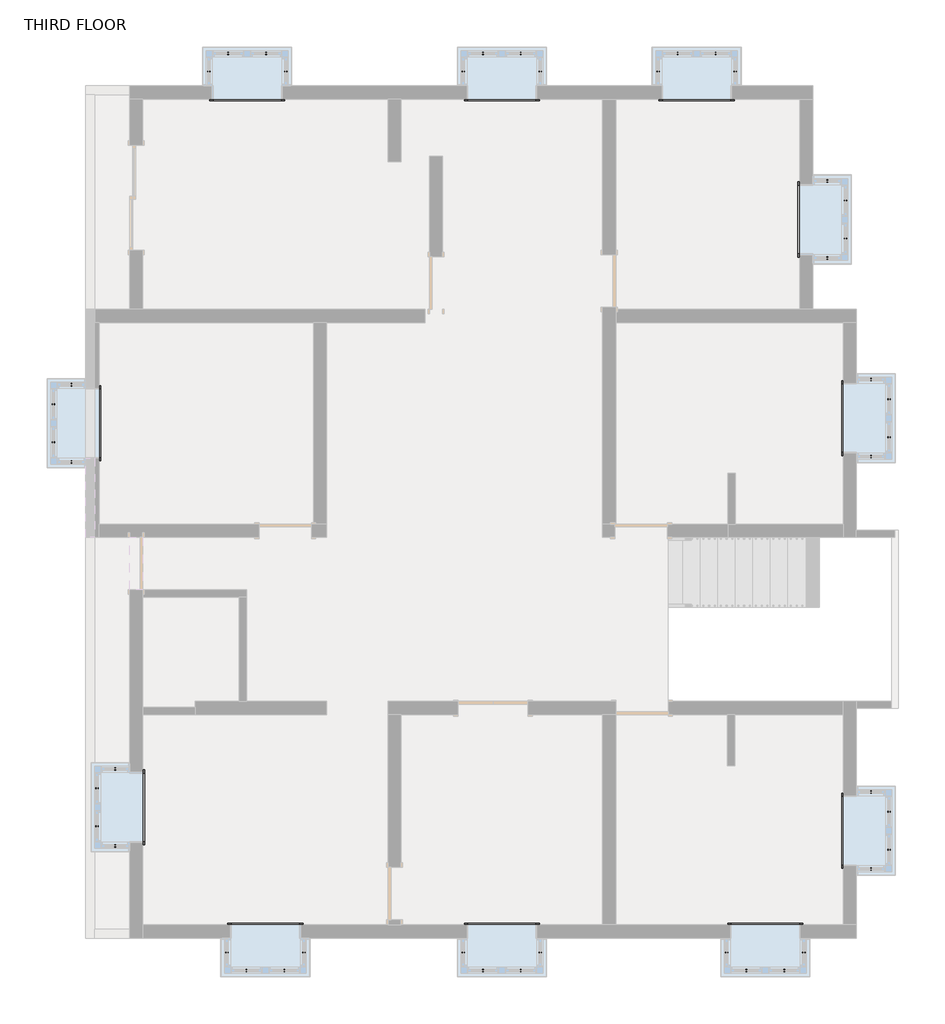
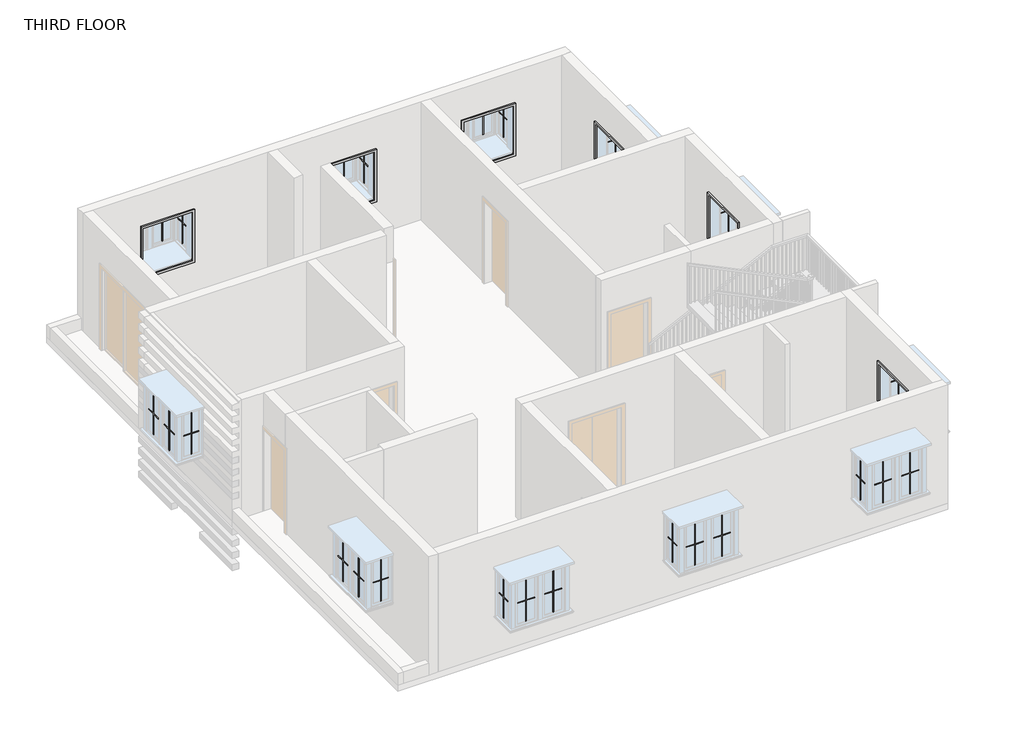
# One storey, part 4 of 4: 55 proxies.
"""IFC4 building model written with IfcOpenShell, lengths in millimetres."""

from ifc_helpers import new_model, si_unit, origin, place, context, project, spatial, transform, mapped, element, save
from components import muntin_pattern_2x2_muntin_pattern_2x2_4aee108e, muntin_pattern_2x2_muntin_pattern_2x2_f03ab90d, muntin_pattern_2x2_muntin_pattern_2x2_eb08c668, trim_window_interior_flat_picture_frame_ace0ae79

model = new_model("IFC4")

# Units and contexts
model_context = context("Model", 3, world=origin())
ifc_project = project(units=[si_unit("LENGTHUNIT", "METRE", prefix="MILLI")], contexts=[model_context])

# Site, building, storey
site = spatial("IfcSite", under=ifc_project)
building = spatial("IfcBuilding", under=site)
storey = spatial("IfcBuildingStorey", under=building, Name="THIRD FLOOR", Elevation=9601.2)

# Proxies
placement = place(None, origin())
muntin_pattern_2x2_muntin_pattern_2x2_shape = muntin_pattern_2x2_muntin_pattern_2x2_4aee108e(model_context)
element("IfcBuildingElementProxy", 1, Name="Muntin Pattern_2x2 : Muntin Pattern_2x2", ObjectType="Muntin Pattern_2x2 : Muntin Pattern_2x2", at=placement, inside=storey, context=model_context, shape_type="MappedRepresentation", body=[
    mapped(muntin_pattern_2x2_muntin_pattern_2x2_shape, transform((6209.1834916, 6075.433346, 10636.25), x_axis=(0.0, -1.0, 0.0), y_axis=(1.0, 0.0, 0.0), z_axis=(0.0, 0.0, 1.0))),
])
element("IfcBuildingElementProxy", 2, Name="Muntin Pattern_2x2 : Muntin Pattern_2x2", ObjectType="Muntin Pattern_2x2 : Muntin Pattern_2x2", at=placement, inside=storey, context=model_context, shape_type="MappedRepresentation", body=[
    mapped(muntin_pattern_2x2_muntin_pattern_2x2_shape, transform((-99.5415084, 8637.658346, 10636.25), x_axis=(1.0, 0.0, 0.0), y_axis=(0.0, 1.0, 0.0), z_axis=(0.0, 0.0, 1.0))),
])
element("IfcBuildingElementProxy", 3, Name="Muntin Pattern_2x2 : Muntin Pattern_2x2", ObjectType="Muntin Pattern_2x2 : Muntin Pattern_2x2", at=placement, inside=storey, context=model_context, shape_type="MappedRepresentation", body=[
    mapped(muntin_pattern_2x2_muntin_pattern_2x2_shape, transform((3291.3584916, 8637.658346, 10636.25), x_axis=(1.0, 0.0, 0.0), y_axis=(0.0, 1.0, 0.0), z_axis=(0.0, 0.0, 1.0))),
])
element("IfcBuildingElementProxy", 4, Name="Muntin Pattern_2x2 : Muntin Pattern_2x2", ObjectType="Muntin Pattern_2x2 : Muntin Pattern_2x2", at=placement, inside=storey, context=model_context, shape_type="MappedRepresentation", body=[
    mapped(muntin_pattern_2x2_muntin_pattern_2x2_shape, transform((-4531.8415084, 8637.658346, 10636.25), x_axis=(1.0, 0.0, 0.0), y_axis=(0.0, 1.0, 0.0), z_axis=(0.0, 0.0, 1.0))),
])
element("IfcBuildingElementProxy", 5, Name="Muntin Pattern_2x2 : Muntin Pattern_2x2", ObjectType="Muntin Pattern_2x2 : Muntin Pattern_2x2", at=placement, inside=storey, context=model_context, shape_type="MappedRepresentation", body=[
    mapped(muntin_pattern_2x2_muntin_pattern_2x2_shape, transform((-7576.6665084, 1871.733346, 10636.25), x_axis=(0.0, 1.0, 0.0), y_axis=(-1.0, 0.0, 0.0), z_axis=(0.0, 0.0, 1.0))),
])
element("IfcBuildingElementProxy", 6, Name="Muntin Pattern_2x2 : Muntin Pattern_2x2", ObjectType="Muntin Pattern_2x2 : Muntin Pattern_2x2", at=placement, inside=storey, context=model_context, shape_type="MappedRepresentation", body=[
    mapped(muntin_pattern_2x2_muntin_pattern_2x2_shape, transform((6971.1834916, 2621.033346, 10636.25), x_axis=(0.0, -1.0, 0.0), y_axis=(1.0, 0.0, 0.0), z_axis=(0.0, 0.0, 1.0))),
])
element("IfcBuildingElementProxy", 7, Name="Muntin Pattern_2x2 : Muntin Pattern_2x2", ObjectType="Muntin Pattern_2x2 : Muntin Pattern_2x2", at=placement, inside=storey, context=model_context, shape_type="MappedRepresentation", body=[
    mapped(muntin_pattern_2x2_muntin_pattern_2x2_shape, transform((-3553.9415084, -7319.891654, 10636.25), x_axis=(-1.0, 0.0, 0.0), y_axis=(0.0, -1.0, 0.0), z_axis=(0.0, 0.0, 1.0))),
])
element("IfcBuildingElementProxy", 8, Name="Muntin Pattern_2x2 : Muntin Pattern_2x2", ObjectType="Muntin Pattern_2x2 : Muntin Pattern_2x2", at=placement, inside=storey, context=model_context, shape_type="MappedRepresentation", body=[
    mapped(muntin_pattern_2x2_muntin_pattern_2x2_shape, transform((5145.5584916, -7319.891654, 10636.25), x_axis=(-1.0, 0.0, 0.0), y_axis=(0.0, -1.0, 0.0), z_axis=(0.0, 0.0, 1.0))),
])
element("IfcBuildingElementProxy", 9, Name="Muntin Pattern_2x2 : Muntin Pattern_2x2", ObjectType="Muntin Pattern_2x2 : Muntin Pattern_2x2", at=placement, inside=storey, context=model_context, shape_type="MappedRepresentation", body=[
    mapped(muntin_pattern_2x2_muntin_pattern_2x2_shape, transform((560.8584916, -7319.891654, 10636.25), x_axis=(-1.0, 0.0, 0.0), y_axis=(0.0, -1.0, 0.0), z_axis=(0.0, 0.0, 1.0))),
])
element("IfcBuildingElementProxy", 10, Name="Muntin Pattern_2x2 : Muntin Pattern_2x2", ObjectType="Muntin Pattern_2x2 : Muntin Pattern_2x2", at=placement, inside=storey, context=model_context, shape_type="MappedRepresentation", body=[
    mapped(muntin_pattern_2x2_muntin_pattern_2x2_shape, transform((-6814.6665084, -4808.466654, 10636.25), x_axis=(0.0, 1.0, 0.0), y_axis=(-1.0, 0.0, 0.0), z_axis=(0.0, 0.0, 1.0))),
])
element("IfcBuildingElementProxy", 11, Name="Muntin Pattern_2x2 : Muntin Pattern_2x2", ObjectType="Muntin Pattern_2x2 : Muntin Pattern_2x2", at=placement, inside=storey, context=model_context, shape_type="MappedRepresentation", body=[
    mapped(muntin_pattern_2x2_muntin_pattern_2x2_shape, transform((6971.1834916, -4554.466654, 10636.25), x_axis=(0.0, -1.0, 0.0), y_axis=(1.0, 0.0, 0.0), z_axis=(0.0, 0.0, 1.0))),
])
muntin_pattern_2x2_muntin_pattern_2x2_2_shape = muntin_pattern_2x2_muntin_pattern_2x2_f03ab90d(model_context)
element("IfcBuildingElementProxy", 12, Name="Muntin Pattern_2x2 : Muntin Pattern_2x2", ObjectType="Muntin Pattern_2x2 : Muntin Pattern_2x2", at=placement, inside=storey, context=model_context, shape_type="MappedRepresentation", body=[
    mapped(muntin_pattern_2x2_muntin_pattern_2x2_2_shape, transform((5894.8584916, 6415.158346, 10636.25), x_axis=(-1.0, 0.0, 0.0), y_axis=(0.0, -1.0, 0.0), z_axis=(0.0, 0.0, 1.0))),
])
element("IfcBuildingElementProxy", 13, Name="Muntin Pattern_2x2 : Muntin Pattern_2x2", ObjectType="Muntin Pattern_2x2 : Muntin Pattern_2x2", at=placement, inside=storey, context=model_context, shape_type="MappedRepresentation", body=[
    mapped(muntin_pattern_2x2_muntin_pattern_2x2_2_shape, transform((5894.8584916, 5075.308346, 10636.25), x_axis=(1.0, 0.0, 0.0), y_axis=(0.0, 1.0, 0.0), z_axis=(0.0, 0.0, 1.0))),
])
element("IfcBuildingElementProxy", 14, Name="Muntin Pattern_2x2 : Muntin Pattern_2x2", ObjectType="Muntin Pattern_2x2 : Muntin Pattern_2x2", at=placement, inside=storey, context=model_context, shape_type="MappedRepresentation", body=[
    mapped(muntin_pattern_2x2_muntin_pattern_2x2_2_shape, transform((-439.2665084, 8323.333346, 10636.25), x_axis=(0.0, -1.0, 0.0), y_axis=(1.0, 0.0, 0.0), z_axis=(0.0, 0.0, 1.0))),
])
element("IfcBuildingElementProxy", 15, Name="Muntin Pattern_2x2 : Muntin Pattern_2x2", ObjectType="Muntin Pattern_2x2 : Muntin Pattern_2x2", at=placement, inside=storey, context=model_context, shape_type="MappedRepresentation", body=[
    mapped(muntin_pattern_2x2_muntin_pattern_2x2_2_shape, transform((900.5834916, 8323.333346, 10636.25), x_axis=(0.0, 1.0, 0.0), y_axis=(-1.0, 0.0, 0.0), z_axis=(0.0, 0.0, 1.0))),
])
element("IfcBuildingElementProxy", 16, Name="Muntin Pattern_2x2 : Muntin Pattern_2x2", ObjectType="Muntin Pattern_2x2 : Muntin Pattern_2x2", at=placement, inside=storey, context=model_context, shape_type="MappedRepresentation", body=[
    mapped(muntin_pattern_2x2_muntin_pattern_2x2_2_shape, transform((2951.6334916, 8323.333346, 10636.25), x_axis=(0.0, -1.0, 0.0), y_axis=(1.0, 0.0, 0.0), z_axis=(0.0, 0.0, 1.0))),
])
element("IfcBuildingElementProxy", 17, Name="Muntin Pattern_2x2 : Muntin Pattern_2x2", ObjectType="Muntin Pattern_2x2 : Muntin Pattern_2x2", at=placement, inside=storey, context=model_context, shape_type="MappedRepresentation", body=[
    mapped(muntin_pattern_2x2_muntin_pattern_2x2_2_shape, transform((4291.4834916, 8323.333346, 10636.25), x_axis=(0.0, 1.0, 0.0), y_axis=(-1.0, 0.0, 0.0), z_axis=(0.0, 0.0, 1.0))),
])
element("IfcBuildingElementProxy", 18, Name="Muntin Pattern_2x2 : Muntin Pattern_2x2", ObjectType="Muntin Pattern_2x2 : Muntin Pattern_2x2", at=placement, inside=storey, context=model_context, shape_type="MappedRepresentation", body=[
    mapped(muntin_pattern_2x2_muntin_pattern_2x2_2_shape, transform((-4871.5665084, 8323.333346, 10636.25), x_axis=(0.0, -1.0, 0.0), y_axis=(1.0, 0.0, 0.0), z_axis=(0.0, 0.0, 1.0))),
])
element("IfcBuildingElementProxy", 19, Name="Muntin Pattern_2x2 : Muntin Pattern_2x2", ObjectType="Muntin Pattern_2x2 : Muntin Pattern_2x2", at=placement, inside=storey, context=model_context, shape_type="MappedRepresentation", body=[
    mapped(muntin_pattern_2x2_muntin_pattern_2x2_2_shape, transform((-3531.7165084, 8323.333346, 10636.25), x_axis=(0.0, 1.0, 0.0), y_axis=(-1.0, 0.0, 0.0), z_axis=(0.0, 0.0, 1.0))),
])
element("IfcBuildingElementProxy", 20, Name="Muntin Pattern_2x2 : Muntin Pattern_2x2", ObjectType="Muntin Pattern_2x2 : Muntin Pattern_2x2", at=placement, inside=storey, context=model_context, shape_type="MappedRepresentation", body=[
    mapped(muntin_pattern_2x2_muntin_pattern_2x2_2_shape, transform((-7262.3415084, 1532.008346, 10636.25), x_axis=(1.0, 0.0, 0.0), y_axis=(0.0, 1.0, 0.0), z_axis=(0.0, 0.0, 1.0))),
])
element("IfcBuildingElementProxy", 21, Name="Muntin Pattern_2x2 : Muntin Pattern_2x2", ObjectType="Muntin Pattern_2x2 : Muntin Pattern_2x2", at=placement, inside=storey, context=model_context, shape_type="MappedRepresentation", body=[
    mapped(muntin_pattern_2x2_muntin_pattern_2x2_2_shape, transform((-7262.3415084, 2871.858346, 10636.25), x_axis=(-1.0, 0.0, 0.0), y_axis=(0.0, -1.0, 0.0), z_axis=(0.0, 0.0, 1.0))),
])
element("IfcBuildingElementProxy", 22, Name="Muntin Pattern_2x2 : Muntin Pattern_2x2", ObjectType="Muntin Pattern_2x2 : Muntin Pattern_2x2", at=placement, inside=storey, context=model_context, shape_type="MappedRepresentation", body=[
    mapped(muntin_pattern_2x2_muntin_pattern_2x2_2_shape, transform((6656.8584916, 2960.758346, 10636.25), x_axis=(-1.0, 0.0, 0.0), y_axis=(0.0, -1.0, 0.0), z_axis=(0.0, 0.0, 1.0))),
])
element("IfcBuildingElementProxy", 23, Name="Muntin Pattern_2x2 : Muntin Pattern_2x2", ObjectType="Muntin Pattern_2x2 : Muntin Pattern_2x2", at=placement, inside=storey, context=model_context, shape_type="MappedRepresentation", body=[
    mapped(muntin_pattern_2x2_muntin_pattern_2x2_2_shape, transform((6656.8584916, 1620.908346, 10636.25), x_axis=(1.0, 0.0, 0.0), y_axis=(0.0, 1.0, 0.0), z_axis=(0.0, 0.0, 1.0))),
])
element("IfcBuildingElementProxy", 24, Name="Muntin Pattern_2x2 : Muntin Pattern_2x2", ObjectType="Muntin Pattern_2x2 : Muntin Pattern_2x2", at=placement, inside=storey, context=model_context, shape_type="MappedRepresentation", body=[
    mapped(muntin_pattern_2x2_muntin_pattern_2x2_2_shape, transform((-3214.2165084, -7005.566654, 10636.25), x_axis=(0.0, 1.0, 0.0), y_axis=(-1.0, 0.0, 0.0), z_axis=(0.0, 0.0, 1.0))),
])
element("IfcBuildingElementProxy", 25, Name="Muntin Pattern_2x2 : Muntin Pattern_2x2", ObjectType="Muntin Pattern_2x2 : Muntin Pattern_2x2", at=placement, inside=storey, context=model_context, shape_type="MappedRepresentation", body=[
    mapped(muntin_pattern_2x2_muntin_pattern_2x2_2_shape, transform((-4554.0665084, -7005.566654, 10636.25), x_axis=(0.0, -1.0, 0.0), y_axis=(1.0, 0.0, 0.0), z_axis=(0.0, 0.0, 1.0))),
])
element("IfcBuildingElementProxy", 26, Name="Muntin Pattern_2x2 : Muntin Pattern_2x2", ObjectType="Muntin Pattern_2x2 : Muntin Pattern_2x2", at=placement, inside=storey, context=model_context, shape_type="MappedRepresentation", body=[
    mapped(muntin_pattern_2x2_muntin_pattern_2x2_2_shape, transform((5485.2834916, -7005.566654, 10636.25), x_axis=(0.0, 1.0, 0.0), y_axis=(-1.0, 0.0, 0.0), z_axis=(0.0, 0.0, 1.0))),
])
element("IfcBuildingElementProxy", 27, Name="Muntin Pattern_2x2 : Muntin Pattern_2x2", ObjectType="Muntin Pattern_2x2 : Muntin Pattern_2x2", at=placement, inside=storey, context=model_context, shape_type="MappedRepresentation", body=[
    mapped(muntin_pattern_2x2_muntin_pattern_2x2_2_shape, transform((4145.4334916, -7005.566654, 10636.25), x_axis=(0.0, -1.0, 0.0), y_axis=(1.0, 0.0, 0.0), z_axis=(0.0, 0.0, 1.0))),
])
element("IfcBuildingElementProxy", 28, Name="Muntin Pattern_2x2 : Muntin Pattern_2x2", ObjectType="Muntin Pattern_2x2 : Muntin Pattern_2x2", at=placement, inside=storey, context=model_context, shape_type="MappedRepresentation", body=[
    mapped(muntin_pattern_2x2_muntin_pattern_2x2_2_shape, transform((900.5834916, -7005.566654, 10636.25), x_axis=(0.0, 1.0, 0.0), y_axis=(-1.0, 0.0, 0.0), z_axis=(0.0, 0.0, 1.0))),
])
element("IfcBuildingElementProxy", 29, Name="Muntin Pattern_2x2 : Muntin Pattern_2x2", ObjectType="Muntin Pattern_2x2 : Muntin Pattern_2x2", at=placement, inside=storey, context=model_context, shape_type="MappedRepresentation", body=[
    mapped(muntin_pattern_2x2_muntin_pattern_2x2_2_shape, transform((-439.2665084, -7005.566654, 10636.25), x_axis=(0.0, -1.0, 0.0), y_axis=(1.0, 0.0, 0.0), z_axis=(0.0, 0.0, 1.0))),
])
element("IfcBuildingElementProxy", 30, Name="Muntin Pattern_2x2 : Muntin Pattern_2x2", ObjectType="Muntin Pattern_2x2 : Muntin Pattern_2x2", at=placement, inside=storey, context=model_context, shape_type="MappedRepresentation", body=[
    mapped(muntin_pattern_2x2_muntin_pattern_2x2_2_shape, transform((-6500.3415084, -5148.191654, 10636.25), x_axis=(1.0, 0.0, 0.0), y_axis=(0.0, 1.0, 0.0), z_axis=(0.0, 0.0, 1.0))),
])
element("IfcBuildingElementProxy", 31, Name="Muntin Pattern_2x2 : Muntin Pattern_2x2", ObjectType="Muntin Pattern_2x2 : Muntin Pattern_2x2", at=placement, inside=storey, context=model_context, shape_type="MappedRepresentation", body=[
    mapped(muntin_pattern_2x2_muntin_pattern_2x2_2_shape, transform((-6500.3415084, -3808.341654, 10636.25), x_axis=(-1.0, 0.0, 0.0), y_axis=(0.0, -1.0, 0.0), z_axis=(0.0, 0.0, 1.0))),
])
element("IfcBuildingElementProxy", 32, Name="Muntin Pattern_2x2 : Muntin Pattern_2x2", ObjectType="Muntin Pattern_2x2 : Muntin Pattern_2x2", at=placement, inside=storey, context=model_context, shape_type="MappedRepresentation", body=[
    mapped(muntin_pattern_2x2_muntin_pattern_2x2_2_shape, transform((6656.8584916, -4214.741654, 10636.25), x_axis=(-1.0, 0.0, 0.0), y_axis=(0.0, -1.0, 0.0), z_axis=(0.0, 0.0, 1.0))),
])
element("IfcBuildingElementProxy", 33, Name="Muntin Pattern_2x2 : Muntin Pattern_2x2", ObjectType="Muntin Pattern_2x2 : Muntin Pattern_2x2", at=placement, inside=storey, context=model_context, shape_type="MappedRepresentation", body=[
    mapped(muntin_pattern_2x2_muntin_pattern_2x2_2_shape, transform((6656.8584916, -5554.591654, 10636.25), x_axis=(1.0, 0.0, 0.0), y_axis=(0.0, 1.0, 0.0), z_axis=(0.0, 0.0, 1.0))),
])
muntin_pattern_2x2_muntin_pattern_2x2_3_shape = muntin_pattern_2x2_muntin_pattern_2x2_eb08c668(model_context)
element("IfcBuildingElementProxy", 34, Name="Muntin Pattern_2x2 : Muntin Pattern_2x2", ObjectType="Muntin Pattern_2x2 : Muntin Pattern_2x2", at=placement, inside=storey, context=model_context, shape_type="MappedRepresentation", body=[
    mapped(muntin_pattern_2x2_muntin_pattern_2x2_3_shape, transform((6209.1834916, 5415.033346, 10636.25), x_axis=(0.0, 1.0, 0.0), y_axis=(-1.0, 0.0, 0.0), z_axis=(0.0, 0.0, 1.0))),
])
element("IfcBuildingElementProxy", 35, Name="Muntin Pattern_2x2 : Muntin Pattern_2x2", ObjectType="Muntin Pattern_2x2 : Muntin Pattern_2x2", at=placement, inside=storey, context=model_context, shape_type="MappedRepresentation", body=[
    mapped(muntin_pattern_2x2_muntin_pattern_2x2_3_shape, transform((560.8584916, 8637.658346, 10636.25), x_axis=(-1.0, 0.0, 0.0), y_axis=(0.0, -1.0, 0.0), z_axis=(0.0, 0.0, 1.0))),
])
element("IfcBuildingElementProxy", 36, Name="Muntin Pattern_2x2 : Muntin Pattern_2x2", ObjectType="Muntin Pattern_2x2 : Muntin Pattern_2x2", at=placement, inside=storey, context=model_context, shape_type="MappedRepresentation", body=[
    mapped(muntin_pattern_2x2_muntin_pattern_2x2_3_shape, transform((3951.7584916, 8637.658346, 10636.25), x_axis=(-1.0, 0.0, 0.0), y_axis=(0.0, -1.0, 0.0), z_axis=(0.0, 0.0, 1.0))),
])
element("IfcBuildingElementProxy", 37, Name="Muntin Pattern_2x2 : Muntin Pattern_2x2", ObjectType="Muntin Pattern_2x2 : Muntin Pattern_2x2", at=placement, inside=storey, context=model_context, shape_type="MappedRepresentation", body=[
    mapped(muntin_pattern_2x2_muntin_pattern_2x2_3_shape, transform((-3871.4415084, 8637.658346, 10636.25), x_axis=(-1.0, 0.0, 0.0), y_axis=(0.0, -1.0, 0.0), z_axis=(0.0, 0.0, 1.0))),
])
element("IfcBuildingElementProxy", 38, Name="Muntin Pattern_2x2 : Muntin Pattern_2x2", ObjectType="Muntin Pattern_2x2 : Muntin Pattern_2x2", at=placement, inside=storey, context=model_context, shape_type="MappedRepresentation", body=[
    mapped(muntin_pattern_2x2_muntin_pattern_2x2_3_shape, transform((-7576.6665084, 2532.133346, 10636.25), x_axis=(0.0, -1.0, 0.0), y_axis=(1.0, 0.0, 0.0), z_axis=(0.0, 0.0, 1.0))),
])
element("IfcBuildingElementProxy", 39, Name="Muntin Pattern_2x2 : Muntin Pattern_2x2", ObjectType="Muntin Pattern_2x2 : Muntin Pattern_2x2", at=placement, inside=storey, context=model_context, shape_type="MappedRepresentation", body=[
    mapped(muntin_pattern_2x2_muntin_pattern_2x2_3_shape, transform((6971.1834916, 1960.633346, 10636.25), x_axis=(0.0, 1.0, 0.0), y_axis=(-1.0, 0.0, 0.0), z_axis=(0.0, 0.0, 1.0))),
])
element("IfcBuildingElementProxy", 40, Name="Muntin Pattern_2x2 : Muntin Pattern_2x2", ObjectType="Muntin Pattern_2x2 : Muntin Pattern_2x2", at=placement, inside=storey, context=model_context, shape_type="MappedRepresentation", body=[
    mapped(muntin_pattern_2x2_muntin_pattern_2x2_3_shape, transform((-4214.3415084, -7319.891654, 10636.25), x_axis=(1.0, 0.0, 0.0), y_axis=(0.0, 1.0, 0.0), z_axis=(0.0, 0.0, 1.0))),
])
element("IfcBuildingElementProxy", 41, Name="Muntin Pattern_2x2 : Muntin Pattern_2x2", ObjectType="Muntin Pattern_2x2 : Muntin Pattern_2x2", at=placement, inside=storey, context=model_context, shape_type="MappedRepresentation", body=[
    mapped(muntin_pattern_2x2_muntin_pattern_2x2_3_shape, transform((4485.1584916, -7319.891654, 10636.25), x_axis=(1.0, 0.0, 0.0), y_axis=(0.0, 1.0, 0.0), z_axis=(0.0, 0.0, 1.0))),
])
element("IfcBuildingElementProxy", 42, Name="Muntin Pattern_2x2 : Muntin Pattern_2x2", ObjectType="Muntin Pattern_2x2 : Muntin Pattern_2x2", at=placement, inside=storey, context=model_context, shape_type="MappedRepresentation", body=[
    mapped(muntin_pattern_2x2_muntin_pattern_2x2_3_shape, transform((-99.5415084, -7319.891654, 10636.25), x_axis=(1.0, 0.0, 0.0), y_axis=(0.0, 1.0, 0.0), z_axis=(0.0, 0.0, 1.0))),
])
element("IfcBuildingElementProxy", 43, Name="Muntin Pattern_2x2 : Muntin Pattern_2x2", ObjectType="Muntin Pattern_2x2 : Muntin Pattern_2x2", at=placement, inside=storey, context=model_context, shape_type="MappedRepresentation", body=[
    mapped(muntin_pattern_2x2_muntin_pattern_2x2_3_shape, transform((-6814.6665084, -4148.066654, 10636.25), x_axis=(0.0, -1.0, 0.0), y_axis=(1.0, 0.0, 0.0), z_axis=(0.0, 0.0, 1.0))),
])
element("IfcBuildingElementProxy", 44, Name="Muntin Pattern_2x2 : Muntin Pattern_2x2", ObjectType="Muntin Pattern_2x2 : Muntin Pattern_2x2", at=placement, inside=storey, context=model_context, shape_type="MappedRepresentation", body=[
    mapped(muntin_pattern_2x2_muntin_pattern_2x2_3_shape, transform((6971.1834916, -5214.866654, 10636.25), x_axis=(0.0, 1.0, 0.0), y_axis=(-1.0, 0.0, 0.0), z_axis=(0.0, 0.0, 1.0))),
])
trim_window_interior_flat_picture_frame_shape = trim_window_interior_flat_picture_frame_ace0ae79(model_context)
element("IfcBuildingElementProxy", 45, Name="Trim-Window-Interior-Flat : Picture Frame", ObjectType="Trim-Window-Interior-Flat : Picture Frame", at=placement, inside=storey, context=model_context, shape_type="MappedRepresentation", body=[
    mapped(trim_window_interior_flat_picture_frame_shape, transform((5412.2584916, 5745.233346, 11785.6), x_axis=(0.0, -1.0, 0.0), y_axis=(0.0, 0.0, 1.0), z_axis=(-1.0, 0.0, 0.0))),
])
element("IfcBuildingElementProxy", 46, Name="Trim-Window-Interior-Flat : Picture Frame", ObjectType="Trim-Window-Interior-Flat : Picture Frame", at=placement, inside=storey, context=model_context, shape_type="MappedRepresentation", body=[
    mapped(trim_window_interior_flat_picture_frame_shape, transform((230.6584916, 7840.733346, 11785.6), x_axis=(1.0, 0.0, 0.0), y_axis=(0.0, 0.0, 1.0), z_axis=(0.0, -1.0, 0.0))),
])
element("IfcBuildingElementProxy", 47, Name="Trim-Window-Interior-Flat : Picture Frame", ObjectType="Trim-Window-Interior-Flat : Picture Frame", at=placement, inside=storey, context=model_context, shape_type="MappedRepresentation", body=[
    mapped(trim_window_interior_flat_picture_frame_shape, transform((3621.5584916, 7840.733346, 11785.6), x_axis=(1.0, 0.0, 0.0), y_axis=(0.0, 0.0, 1.0), z_axis=(0.0, -1.0, 0.0))),
])
element("IfcBuildingElementProxy", 48, Name="Trim-Window-Interior-Flat : Picture Frame", ObjectType="Trim-Window-Interior-Flat : Picture Frame", at=placement, inside=storey, context=model_context, shape_type="MappedRepresentation", body=[
    mapped(trim_window_interior_flat_picture_frame_shape, transform((-4201.6415084, 7840.733346, 11785.6), x_axis=(1.0, 0.0, 0.0), y_axis=(0.0, 0.0, 1.0), z_axis=(0.0, -1.0, 0.0))),
])
element("IfcBuildingElementProxy", 49, Name="Trim-Window-Interior-Flat : Picture Frame", ObjectType="Trim-Window-Interior-Flat : Picture Frame", at=placement, inside=storey, context=model_context, shape_type="MappedRepresentation", body=[
    mapped(trim_window_interior_flat_picture_frame_shape, transform((-6779.7415084, 2201.933346, 11785.6), x_axis=(0.0, 1.0, 0.0), y_axis=(0.0, 0.0, 1.0), z_axis=(1.0, 0.0, 0.0))),
])
element("IfcBuildingElementProxy", 50, Name="Trim-Window-Interior-Flat : Picture Frame", ObjectType="Trim-Window-Interior-Flat : Picture Frame", at=placement, inside=storey, context=model_context, shape_type="MappedRepresentation", body=[
    mapped(trim_window_interior_flat_picture_frame_shape, transform((6174.2584916, 2290.833346, 11785.6), x_axis=(0.0, -1.0, 0.0), y_axis=(0.0, 0.0, 1.0), z_axis=(-1.0, 0.0, 0.0))),
])
element("IfcBuildingElementProxy", 51, Name="Trim-Window-Interior-Flat : Picture Frame", ObjectType="Trim-Window-Interior-Flat : Picture Frame", at=placement, inside=storey, context=model_context, shape_type="MappedRepresentation", body=[
    mapped(trim_window_interior_flat_picture_frame_shape, transform((-3884.1415084, -6522.966654, 11785.6), x_axis=(-1.0, 0.0, 0.0), y_axis=(0.0, 0.0, 1.0), z_axis=(0.0, 1.0, 0.0))),
])
element("IfcBuildingElementProxy", 52, Name="Trim-Window-Interior-Flat : Picture Frame", ObjectType="Trim-Window-Interior-Flat : Picture Frame", at=placement, inside=storey, context=model_context, shape_type="MappedRepresentation", body=[
    mapped(trim_window_interior_flat_picture_frame_shape, transform((4815.3584916, -6522.966654, 11785.6), x_axis=(-1.0, 0.0, 0.0), y_axis=(0.0, 0.0, 1.0), z_axis=(0.0, 1.0, 0.0))),
])
element("IfcBuildingElementProxy", 53, Name="Trim-Window-Interior-Flat : Picture Frame", ObjectType="Trim-Window-Interior-Flat : Picture Frame", at=placement, inside=storey, context=model_context, shape_type="MappedRepresentation", body=[
    mapped(trim_window_interior_flat_picture_frame_shape, transform((230.6584916, -6522.966654, 11785.6), x_axis=(-1.0, 0.0, 0.0), y_axis=(0.0, 0.0, 1.0), z_axis=(0.0, 1.0, 0.0))),
])
element("IfcBuildingElementProxy", 54, Name="Trim-Window-Interior-Flat : Picture Frame", ObjectType="Trim-Window-Interior-Flat : Picture Frame", at=placement, inside=storey, context=model_context, shape_type="MappedRepresentation", body=[
    mapped(trim_window_interior_flat_picture_frame_shape, transform((-6017.7415084, -4478.266654, 11785.6), x_axis=(0.0, 1.0, 0.0), y_axis=(0.0, 0.0, 1.0), z_axis=(1.0, 0.0, 0.0))),
])
element("IfcBuildingElementProxy", 55, Name="Trim-Window-Interior-Flat : Picture Frame", ObjectType="Trim-Window-Interior-Flat : Picture Frame", at=placement, inside=storey, context=model_context, shape_type="MappedRepresentation", body=[
    mapped(trim_window_interior_flat_picture_frame_shape, transform((6174.2584916, -4884.666654, 11785.6), x_axis=(0.0, -1.0, 0.0), y_axis=(0.0, 0.0, 1.0), z_axis=(-1.0, 0.0, 0.0))),
])

save(model, "model.ifc")

# Revit data of these elements
# Type "Muntin Pattern_2x2 : Muntin Pattern_2x2"
#   Width [instance default] = 4' - 0"
#   Thickness = 0' - 0 1/2"
#   Height [instance default] = 4' - 0"
#   Distance = 0' - 0 3/4"
#   Interior Material [instance default] = none
#   Exterior Material [instance default] = none
#   Default Elevation = 0
# Type "Trim-Window-Interior-Flat : Picture Frame"
#   Trim Thickness_Picture Frame = 0' - 1 1/4"
#   Trim Width = 0' - 2 1/4"
#   Trim Thickness_with Sill = 0' - 0 3/4"
#   Sill Thickness = 0' - 1 1/4"
#   Opening Width [instance default] = 2' - 0"
#   Opening Height [instance default] = 3' - 0"
#   Default Elevation = 4' - 0"
#   Sill = no
#   Picture Frame = yes
#   Trim Material [instance default] = none
# Elements 1, 2, 3, 4, 5, 6, 7, 8, 9, 10, 11, 34, 35, 36, 37, 38, 39, 40, 41, 42, 43, 44 (IfcBuildingElementProxy, "Muntin Pattern_2x2 : Muntin Pattern_2x2")
#   Width = 1' - 4 1/2"
#   Height = 3' - 6 1/2"
#   Interior Material = Wood - Stained
#   Exterior Material = Clad - White
#   Phase Created = New Construction
#   Materials on its faces: "Clad - White", "Wood - Stained"
# Elements 12, 13, 14, 15, 16, 17, 18, 19, 20, 21, 22, 23, 24, 25, 26, 27, 28, 29, 30, 31, 32, 33 (IfcBuildingElementProxy, "Muntin Pattern_2x2 : Muntin Pattern_2x2")
#   Width = 1' - 2 1/2"
#   Height = 3' - 6 1/2"
#   Interior Material = Wood - Stained
#   Exterior Material = Clad - White
#   Phase Created = New Construction
#   Materials on its faces: "Clad - White", "Wood - Stained"
# Elements 45, 46, 47, 48, 49, 50, 51, 52, 53, 54, 55 (IfcBuildingElementProxy, "Trim-Window-Interior-Flat : Picture Frame")
#   Opening Width = 4' - 0"
#   Opening Height = 4' - 2"
#   Trim Material = Wood - Stained
#   Phase Created = New Construction
#   Materials on its faces: "Wood - Stained"
# Materials
#   "Clad - White": class "Wood", colour RGB 242 242 238, transparency 0, Cost = 0
#   "Wood - Stained": class "Wood", colour RGB 224 178 126, transparency 0, Cost = 0
